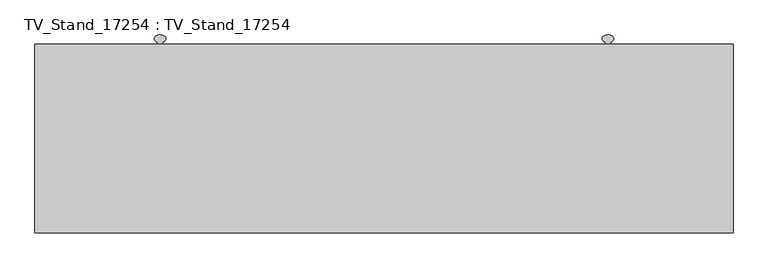
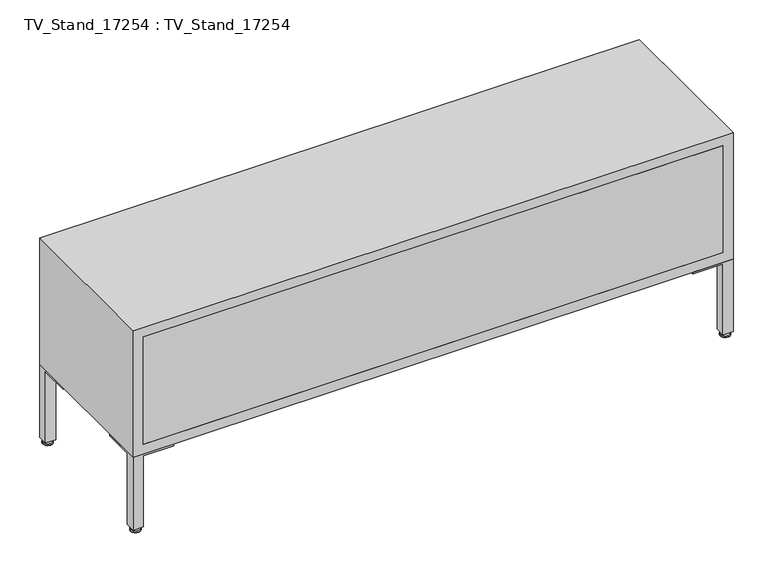
"""IFC4 building model written with IfcOpenShell, lengths in millimetres: furniture geometry, TV_Stand_17254 : TV_Stand_17254."""

from ifc_helpers import new_model, si_unit, point, frame, origin, place, context, project, spatial, polyline, circle_curve, ellipse_curve, trimmed, outline, extrude, source, transform, mapped, element, save
from ifc_brep_helpers import plane_surface, cylinder_surface, revolved_surface, extruded_surface, advanced_brep


def tv_stand_17254_tv_stand_17254_2bb553a4(model_context):
    return source(origin(), model_context, "Body", "SolidModel", [
        extrude(outline(polyline([(530.0, 740.0), (530.0, -740.0), (200.0, -740.0), (200.0, 740.0), (530.0, 740.0)]), holes=[polyline([(505.0, 715.0), (225.0, 715.0), (225.0, -715.0), (505.0, -715.0), (505.0, 715.0)])]), frame((0.0, 0.0, 0.0), z_axis=(0.0, 1.0, 0.0), x_axis=(0.0, 0.0, 1.0)), (0.0, 0.0, 1.0), 400.0),
        extrude(outline(polyline([(-400.0, 12.0), (-412.0, 12.0), (-412.0, 390.0), (-400.0, 390.0), (-400.0, 12.0)])), frame((0.0, 0.0, 225.0), z_axis=(0.0, 0.0, 1.0), x_axis=(1.0, 0.0, 0.0)), (0.0, 0.0, 1.0), 280.0),
        extrude(outline(polyline([(412.0, 12.0), (400.0, 12.0), (400.0, 390.0), (412.0, 390.0), (412.0, 12.0)])), frame((0.0, 0.0, 225.0), z_axis=(0.0, 0.0, 1.0), x_axis=(1.0, 0.0, 0.0)), (0.0, 0.0, 1.0), 280.0),
        extrude(outline(polyline([(715.0, 0.0), (-715.0, 0.0), (-715.0, 12.0), (715.0, 12.0), (715.0, 0.0)])), frame((0.0, 0.0, 225.0), z_axis=(0.0, 0.0, 1.0), x_axis=(1.0, 0.0, 0.0)), (0.0, 0.0, 1.0), 280.0),
        extrude(outline(polyline([(-400.0, 400.0), (-400.0, 390.0), (-713.0, 390.0), (-713.0, 400.0), (-400.0, 400.0)])), frame((0.0, 0.0, 227.0), z_axis=(0.0, 0.0, 1.0), x_axis=(1.0, 0.0, 0.0)), (0.0, 0.0, 1.0), 276.0),
        extrude(outline(polyline([(400.0, 400.0), (713.0, 400.0), (713.0, 390.0), (400.0, 390.0), (400.0, 400.0)])), frame((0.0, 0.0, 227.0), z_axis=(0.0, 0.0, 1.0), x_axis=(1.0, 0.0, 0.0)), (0.0, 0.0, 1.0), 276.0),
        extrude(outline(polyline([(400.0, 12.0), (-400.0, 12.0), (-400.0, 390.0), (400.0, 390.0), (400.0, 12.0)])), frame((0.0, 0.0, 352.5), z_axis=(0.0, 0.0, 1.0), x_axis=(1.0, 0.0, 0.0)), (0.0, 0.0, 1.0), 25.0),
        advanced_brep(
        [(-715.0, 400.0, 10.0), (-715.0, 375.0, 10.0), (-740.0, 375.0, 10.0), (-740.0, 400.0, 10.0), (-730.0, 387.5, 10.0), (-725.0, 387.5, 10.0), (-740.0, 400.0, 200.0), (-640.0, 400.0, 200.0), (-640.0, 400.0, 195.0), (-715.0, 400.0, 195.0), (-740.0, 375.0, 195.0), (-740.0, 300.0, 195.0), (-740.0, 300.0, 200.0), (-715.0, 375.0, 195.0), (-715.0, 300.0, 200.0), (-715.0, 375.0, 200.0), (-640.0, 375.0, 200.0), (-640.0, 375.0, 195.0), (-715.0, 300.0, 195.0), (-730.0, 387.5, 7.0), (-725.0, 387.5, 7.0), (-738.4284767, 387.5, 3.6286093), (-716.5715233, 387.5, 3.6286093), (-740.0, 387.5, 1.3074176), (-715.0, 387.5, 1.3074176), (-740.0, 387.5, 0.0), (-715.0, 387.5, 0.0), (-727.5, 387.5, 0.0)],
        [
            (0, 1),
            (1, 2),
            (2, 3),
            (3, 0),
            (4, 5, circle_curve(frame((-727.5, 387.5, 10.0), z_axis=(0.0, 0.0, 1.0), x_axis=(-1.0, 0.0, 0.0)), 2.5)),
            (5, 4, circle_curve(frame((-727.5, 387.5, 10.0), z_axis=(0.0, 0.0, 1.0), x_axis=(-1.0, 0.0, 0.0)), 2.5)),
            (3, 6),
            (6, 7),
            (7, 8),
            (8, 9),
            (9, 0),
            (2, 10),
            (10, 11),
            (11, 12),
            (12, 6),
            (1, 13),
            (13, 10),
            (9, 13),
            (12, 14),
            (14, 15),
            (15, 16),
            (16, 7),
            (8, 17),
            (17, 13),
            (13, 18),
            (18, 11),
            (18, 14),
            (13, 15),
            (17, 16),
            (4, 19),
            (19, 20, circle_curve(frame((-727.5, 387.5, 7.0), z_axis=(0.0, 0.0, 1.0), x_axis=(-1.0, 0.0, 0.0)), 2.5)),
            (20, 5),
            (20, 19, circle_curve(frame((-727.5, 387.5, 7.0), z_axis=(0.0, 0.0, 1.0), x_axis=(-1.0, 0.0, 0.0)), 2.5)),
            (19, 21),
            (21, 22, circle_curve(frame((-727.5, 387.5, 3.6286093), z_axis=(0.0, 0.0, 1.0), x_axis=(-1.0, 0.0, 0.0)), 10.9284767)),
            (22, 20),
            (22, 21, circle_curve(frame((-727.5, 387.5, 3.6286093), z_axis=(0.0, 0.0, 1.0), x_axis=(-1.0, 0.0, 0.0)), 10.9284767)),
            (21, 23, circle_curve(frame((-737.5, 387.5, 1.3074176), z_axis=(0.0, -1.0, 0.0), x_axis=(1.0, 0.0, 0.0)), 2.5)),
            (23, 24, circle_curve(frame((-727.5, 387.5, 1.3074176), z_axis=(0.0, 0.0, 1.0), x_axis=(-1.0, 0.0, 0.0)), 12.5)),
            (24, 22, circle_curve(frame((-717.5, 387.5, 1.3074176), z_axis=(0.0, -1.0, 0.0), x_axis=(-1.0, 0.0, 0.0)), 2.5)),
            (24, 23, circle_curve(frame((-727.5, 387.5, 1.3074176), z_axis=(0.0, 0.0, 1.0), x_axis=(-1.0, 0.0, 0.0)), 12.5)),
            (23, 25),
            (25, 26, circle_curve(frame((-727.5, 387.5, 0.0), z_axis=(0.0, 0.0, 1.0), x_axis=(-1.0, 0.0, 0.0)), 12.5)),
            (26, 24),
            (26, 25, circle_curve(frame((-727.5, 387.5, 0.0), z_axis=(0.0, 0.0, 1.0), x_axis=(-1.0, 0.0, 0.0)), 12.5)),
            (25, 27),
            (27, 26),
        ],
        [
            plane_surface(frame((-740.0, 400.0, 10.0), z_axis=(0.0, 0.0, -1.0), x_axis=(1.0, 0.0, 0.0))),
            plane_surface(frame((-715.0, 400.0, 195.0), z_axis=(0.0, 1.0, 0.0), x_axis=(0.0, 0.0, -1.0))),
            plane_surface(frame((-740.0, 400.0, 195.0), z_axis=(-1.0, 0.0, 0.0), x_axis=(0.0, 0.0, -1.0))),
            plane_surface(frame((-740.0, 375.0, 195.0), z_axis=(0.0, -1.0, 0.0), x_axis=(0.0, 0.0, -1.0))),
            plane_surface(frame((-715.0, 375.0, 195.0), z_axis=(1.0, 0.0, 0.0), x_axis=(0.0, 0.0, -1.0))),
            plane_surface(frame((-740.0, 300.0, 200.0), z_axis=(0.0, 0.0, 1.0), x_axis=(1.0, 0.0, 0.0))),
            plane_surface(frame((-740.0, 300.0, 195.0), z_axis=(0.0, 0.0, -1.0), x_axis=(-1.0, 0.0, 0.0))),
            plane_surface(frame((-740.0, 300.0, 200.0), z_axis=(0.0, -1.0, 0.0), x_axis=(0.0, 0.0, -1.0))),
            plane_surface(frame((-715.0, 300.0, 200.0), z_axis=(1.0, 0.0, 0.0), x_axis=(0.0, 0.0, -1.0))),
            plane_surface(frame((-715.0, 375.0, 200.0), z_axis=(0.0, -1.0, 0.0), x_axis=(0.0, 0.0, -1.0))),
            plane_surface(frame((-640.0, 375.0, 200.0), z_axis=(1.0, 0.0, 0.0), x_axis=(0.0, 0.0, -1.0))),
            cylinder_surface(frame((-727.5, 387.5, 10.0), z_axis=(0.0, 0.0, 1.0), x_axis=(-1.0, 0.0, 0.0)), 2.5),
            revolved_surface(polyline([(-738.4284767, 387.5, 3.6286093), (-730.0, 387.5, 7.0)]), (-727.5, 387.5, 10.0), (0.0, 0.0, 1.0)),
            revolved_surface(trimmed(ellipse_curve(frame((-737.5, 387.5, 1.3074176), z_axis=(0.0, 1.0, 0.0), x_axis=(1.0, 0.0, 0.0)), 2.5, 2.5), [point((-740.0, 387.5, 1.3074176))], [point((-738.4284767, 387.5, 3.6286093))], True, "CARTESIAN"), (-727.5, 387.5, 10.0), (0.0, 0.0, 1.0)),
            cylinder_surface(frame((-727.5, 387.5, 10.0), z_axis=(0.0, 0.0, 1.0), x_axis=(-1.0, 0.0, 0.0)), 12.5),
            plane_surface(frame((-727.5, 387.5, 0.0), z_axis=(0.0, 0.0, -1.0), x_axis=(-1.0, 0.0, 0.0))),
        ],
        [
            (0, [[1, 2, 3, 4], [5, 6]]),
            (1, [[-4, 7, 8, 9, 10, 11]]),
            (2, [[-3, 12, 13, 14, 15, -7]]),
            (3, [[-2, 16, 17, -12]]),
            (4, [[-1, -11, 18, -16]]),
            (5, [[19, 20, 21, 22, -8, -15]]),
            (6, [[23, 24, -18, -10]]),
            (6, [[25, 26, -13, -17]]),
            (7, [[-19, -14, -26, 27]]),
            (8, [[-20, -27, -25, 28]]),
            (9, [[-21, -28, -24, 29]]),
            (10, [[-22, -29, -23, -9]]),
            (11, [[30, 31, 32, -5]]),
            (11, [[-30, -6, -32, 33]]),
            (12, [[-31, 34, 35, 36]]),
            (12, [[-33, -36, 37, -34]]),
            (13, [[-35, 38, 39, 40]]),
            (13, [[-37, -40, 41, -38]]),
            (14, [[-39, 42, 43, 44]]),
            (14, [[-41, -44, 45, -42]]),
            (15, [[-43, 46, 47]]),
            (15, [[-45, -47, -46]]),
        ],
    ),
        advanced_brep(
        [(-715.0, 0.0, 10.0), (-740.0, 0.0, 10.0), (-740.0, 25.0, 10.0), (-715.0, 25.0, 10.0), (-725.0, 12.5, 10.0), (-730.0, 12.5, 10.0), (-715.0, 25.0, 195.0), (-715.0, 0.0, 195.0), (-740.0, 25.0, 195.0), (-740.0, 0.0, 200.0), (-740.0, 100.0, 200.0), (-740.0, 100.0, 195.0), (-640.0, 0.0, 195.0), (-640.0, 0.0, 200.0), (-640.0, 25.0, 200.0), (-715.0, 25.0, 200.0), (-715.0, 100.0, 200.0), (-715.0, 100.0, 195.0), (-640.0, 25.0, 195.0), (-725.0, 12.5, 7.0), (-730.0, 12.5, 7.0), (-716.5715233, 12.5, 3.6286093), (-738.4284767, 12.5, 3.6286093), (-715.0, 12.5, 1.3074176), (-740.0, 12.5, 1.3074176), (-715.0, 12.5, 0.0), (-740.0, 12.5, 0.0), (-727.5, 12.5, 0.0)],
        [
            (0, 1),
            (1, 2),
            (2, 3),
            (3, 0),
            (4, 5, circle_curve(frame((-727.5, 12.5, 10.0), z_axis=(0.0, 0.0, 1.0), x_axis=(-1.0, 0.0, 0.0)), 2.5)),
            (5, 4, circle_curve(frame((-727.5, 12.5, 10.0), z_axis=(0.0, 0.0, 1.0), x_axis=(-1.0, 0.0, 0.0)), 2.5)),
            (3, 6),
            (6, 7),
            (7, 0),
            (2, 8),
            (8, 6),
            (1, 9),
            (9, 10),
            (10, 11),
            (11, 8),
            (7, 12),
            (12, 13),
            (13, 9),
            (13, 14),
            (14, 15),
            (15, 16),
            (16, 10),
            (11, 17),
            (17, 6),
            (6, 18),
            (18, 12),
            (18, 14),
            (6, 15),
            (17, 16),
            (19, 20, circle_curve(frame((-727.5, 12.5, 7.0), z_axis=(0.0, 0.0, 1.0), x_axis=(-1.0, 0.0, 0.0)), 2.5)),
            (20, 5),
            (4, 19),
            (20, 19, circle_curve(frame((-727.5, 12.5, 7.0), z_axis=(0.0, 0.0, 1.0), x_axis=(-1.0, 0.0, 0.0)), 2.5)),
            (19, 21),
            (21, 22, circle_curve(frame((-727.5, 12.5, 3.6286093), z_axis=(0.0, 0.0, 1.0), x_axis=(-1.0, 0.0, 0.0)), 10.9284767)),
            (22, 20),
            (22, 21, circle_curve(frame((-727.5, 12.5, 3.6286093), z_axis=(0.0, 0.0, 1.0), x_axis=(-1.0, 0.0, 0.0)), 10.9284767)),
            (21, 23, circle_curve(frame((-717.5, 12.5, 1.3074176), z_axis=(0.0, 1.0, 0.0), x_axis=(-1.0, 0.0, 0.0)), 2.5)),
            (23, 24, circle_curve(frame((-727.5, 12.5, 1.3074176), z_axis=(0.0, 0.0, 1.0), x_axis=(-1.0, 0.0, 0.0)), 12.5)),
            (24, 22, circle_curve(frame((-737.5, 12.5, 1.3074176), z_axis=(0.0, 1.0, 0.0), x_axis=(1.0, 0.0, 0.0)), 2.5)),
            (24, 23, circle_curve(frame((-727.5, 12.5, 1.3074176), z_axis=(0.0, 0.0, 1.0), x_axis=(-1.0, 0.0, 0.0)), 12.5)),
            (23, 25),
            (25, 26, circle_curve(frame((-727.5, 12.5, 0.0), z_axis=(0.0, 0.0, 1.0), x_axis=(-1.0, 0.0, 0.0)), 12.5)),
            (26, 24),
            (26, 25, circle_curve(frame((-727.5, 12.5, 0.0), z_axis=(0.0, 0.0, 1.0), x_axis=(-1.0, 0.0, 0.0)), 12.5)),
            (25, 27),
            (27, 26),
        ],
        [
            plane_surface(frame((-740.0, 400.0, 10.0), z_axis=(0.0, 0.0, -1.0), x_axis=(1.0, 0.0, 0.0))),
            plane_surface(frame((-715.0, 0.0, 195.0), z_axis=(1.0, 0.0, 0.0), x_axis=(0.0, 0.0, -1.0))),
            plane_surface(frame((-715.0, 25.0, 195.0), z_axis=(0.0, 1.0, 0.0), x_axis=(0.0, 0.0, -1.0))),
            plane_surface(frame((-740.0, 25.0, 195.0), z_axis=(-1.0, 0.0, 0.0), x_axis=(0.0, 0.0, -1.0))),
            plane_surface(frame((-740.0, 0.0, 195.0), z_axis=(0.0, -1.0, 0.0), x_axis=(0.0, 0.0, -1.0))),
            plane_surface(frame((-740.0, 300.0, 200.0), z_axis=(0.0, 0.0, 1.0), x_axis=(1.0, 0.0, 0.0))),
            plane_surface(frame((-740.0, 300.0, 195.0), z_axis=(0.0, 0.0, -1.0), x_axis=(-1.0, 0.0, 0.0))),
            plane_surface(frame((-640.0, 0.0, 200.0), z_axis=(1.0, 0.0, 0.0), x_axis=(0.0, 0.0, -1.0))),
            plane_surface(frame((-640.0, 25.0, 200.0), z_axis=(0.0, 1.0, 0.0), x_axis=(0.0, 0.0, -1.0))),
            plane_surface(frame((-715.0, 25.0, 200.0), z_axis=(1.0, 0.0, 0.0), x_axis=(0.0, 0.0, -1.0))),
            plane_surface(frame((-715.0, 100.0, 200.0), z_axis=(0.0, 1.0, 0.0), x_axis=(0.0, 0.0, -1.0))),
            cylinder_surface(frame((-727.5, 12.5, 10.0), z_axis=(0.0, 0.0, -1.0), x_axis=(-1.0, 0.0, 0.0)), 2.5),
            revolved_surface(polyline([(-730.0, 12.5, 7.0), (-738.4284767, 12.5, 3.6286093)]), (-727.5, 12.5, 10.0), (0.0, 0.0, -1.0)),
            revolved_surface(trimmed(ellipse_curve(frame((-737.5, 12.5, 1.3074176), z_axis=(0.0, -1.0, 0.0), x_axis=(1.0, 0.0, 0.0)), 2.5, 2.5), [point((-738.4284767, 12.5, 3.6286093))], [point((-740.0, 12.5, 1.3074176))], True, "CARTESIAN"), (-727.5, 12.5, 10.0), (0.0, 0.0, -1.0)),
            cylinder_surface(frame((-727.5, 12.5, 10.0), z_axis=(0.0, 0.0, -1.0), x_axis=(-1.0, 0.0, 0.0)), 12.5),
            plane_surface(frame((-727.5, 12.5, 0.0), z_axis=(0.0, 0.0, -1.0), x_axis=(-1.0, 0.0, 0.0))),
        ],
        [
            (0, [[1, 2, 3, 4], [5, 6]]),
            (1, [[-4, 7, 8, 9]]),
            (2, [[-3, 10, 11, -7]]),
            (3, [[-2, 12, 13, 14, 15, -10]]),
            (4, [[-1, -9, 16, 17, 18, -12]]),
            (5, [[-13, -18, 19, 20, 21, 22]]),
            (6, [[23, 24, -11, -15]]),
            (6, [[25, 26, -16, -8]]),
            (7, [[-19, -17, -26, 27]]),
            (8, [[-20, -27, -25, 28]]),
            (9, [[-21, -28, -24, 29]]),
            (10, [[-22, -29, -23, -14]]),
            (11, [[30, 31, -5, 32]]),
            (11, [[-31, 33, -32, -6]]),
            (12, [[-30, 34, 35, 36]]),
            (12, [[-33, -36, 37, -34]]),
            (13, [[-35, 38, 39, 40]]),
            (13, [[-37, -40, 41, -38]]),
            (14, [[-39, 42, 43, 44]]),
            (14, [[-41, -44, 45, -42]]),
            (15, [[-43, 46, 47]]),
            (15, [[-45, -47, -46]]),
        ],
    ),
        advanced_brep(
        [(715.0, 400.0, 10.0), (740.0, 400.0, 10.0), (740.0, 375.0, 10.0), (715.0, 375.0, 10.0), (725.0, 387.5, 10.0), (730.0, 387.5, 10.0), (715.0, 375.0, 195.0), (715.0, 400.0, 195.0), (740.0, 375.0, 195.0), (740.0, 400.0, 200.0), (740.0, 300.0, 200.0), (740.0, 300.0, 195.0), (640.0, 400.0, 195.0), (640.0, 400.0, 200.0), (640.0, 375.0, 200.0), (715.0, 375.0, 200.0), (715.0, 300.0, 200.0), (715.0, 300.0, 195.0), (640.0, 375.0, 195.0), (725.0, 387.5, 7.0), (730.0, 387.5, 7.0), (716.5715233, 387.5, 3.6286093), (738.4284767, 387.5, 3.6286093), (715.0, 387.5, 1.3074176), (740.0, 387.5, 1.3074176), (715.0, 387.5, 0.0), (740.0, 387.5, 0.0), (727.5, 387.5, 0.0)],
        [
            (0, 1),
            (1, 2),
            (2, 3),
            (3, 0),
            (4, 5, circle_curve(frame((727.5, 387.5, 10.0), z_axis=(0.0, 0.0, 1.0), x_axis=(1.0, 0.0, 0.0)), 2.5)),
            (5, 4, circle_curve(frame((727.5, 387.5, 10.0), z_axis=(0.0, 0.0, 1.0), x_axis=(1.0, 0.0, 0.0)), 2.5)),
            (3, 6),
            (6, 7),
            (7, 0),
            (2, 8),
            (8, 6),
            (1, 9),
            (9, 10),
            (10, 11),
            (11, 8),
            (7, 12),
            (12, 13),
            (13, 9),
            (13, 14),
            (14, 15),
            (15, 16),
            (16, 10),
            (11, 17),
            (17, 6),
            (6, 18),
            (18, 12),
            (18, 14),
            (6, 15),
            (17, 16),
            (19, 20, circle_curve(frame((727.5, 387.5, 7.0), z_axis=(0.0, 0.0, 1.0), x_axis=(1.0, 0.0, 0.0)), 2.5)),
            (20, 5),
            (4, 19),
            (20, 19, circle_curve(frame((727.5, 387.5, 7.0), z_axis=(0.0, 0.0, 1.0), x_axis=(1.0, 0.0, 0.0)), 2.5)),
            (19, 21),
            (21, 22, circle_curve(frame((727.5, 387.5, 3.6286093), z_axis=(0.0, 0.0, 1.0), x_axis=(1.0, 0.0, 0.0)), 10.9284767)),
            (22, 20),
            (22, 21, circle_curve(frame((727.5, 387.5, 3.6286093), z_axis=(0.0, 0.0, 1.0), x_axis=(1.0, 0.0, 0.0)), 10.9284767)),
            (21, 23, circle_curve(frame((717.5, 387.5, 1.3074176), z_axis=(0.0, -1.0, 0.0), x_axis=(1.0, 0.0, 0.0)), 2.5)),
            (23, 24, circle_curve(frame((727.5, 387.5, 1.3074176), z_axis=(0.0, 0.0, 1.0), x_axis=(1.0, 0.0, 0.0)), 12.5)),
            (24, 22, circle_curve(frame((737.5, 387.5, 1.3074176), z_axis=(0.0, -1.0, 0.0), x_axis=(-1.0, 0.0, 0.0)), 2.5)),
            (24, 23, circle_curve(frame((727.5, 387.5, 1.3074176), z_axis=(0.0, 0.0, 1.0), x_axis=(1.0, 0.0, 0.0)), 12.5)),
            (23, 25),
            (25, 26, circle_curve(frame((727.5, 387.5, 0.0), z_axis=(0.0, 0.0, 1.0), x_axis=(1.0, 0.0, 0.0)), 12.5)),
            (26, 24),
            (26, 25, circle_curve(frame((727.5, 387.5, 0.0), z_axis=(0.0, 0.0, 1.0), x_axis=(1.0, 0.0, 0.0)), 12.5)),
            (25, 27),
            (27, 26),
        ],
        [
            plane_surface(frame((-740.0, 400.0, 10.0), z_axis=(0.0, 0.0, -1.0), x_axis=(1.0, 0.0, 0.0))),
            plane_surface(frame((715.0, 400.0, 195.0), z_axis=(-1.0, 0.0, 0.0), x_axis=(0.0, 0.0, -1.0))),
            plane_surface(frame((715.0, 375.0, 195.0), z_axis=(0.0, -1.0, 0.0), x_axis=(0.0, 0.0, -1.0))),
            plane_surface(frame((740.0, 375.0, 195.0), z_axis=(1.0, 0.0, 0.0), x_axis=(0.0, 0.0, -1.0))),
            plane_surface(frame((740.0, 400.0, 195.0), z_axis=(0.0, 1.0, 0.0), x_axis=(0.0, 0.0, -1.0))),
            plane_surface(frame((-740.0, 300.0, 200.0), z_axis=(0.0, 0.0, 1.0), x_axis=(1.0, 0.0, 0.0))),
            plane_surface(frame((-740.0, 300.0, 195.0), z_axis=(0.0, 0.0, -1.0), x_axis=(-1.0, 0.0, 0.0))),
            plane_surface(frame((640.0, 400.0, 200.0), z_axis=(-1.0, 0.0, 0.0), x_axis=(0.0, 0.0, -1.0))),
            plane_surface(frame((640.0, 375.0, 200.0), z_axis=(0.0, -1.0, 0.0), x_axis=(0.0, 0.0, -1.0))),
            plane_surface(frame((715.0, 375.0, 200.0), z_axis=(-1.0, 0.0, 0.0), x_axis=(0.0, 0.0, -1.0))),
            plane_surface(frame((715.0, 300.0, 200.0), z_axis=(0.0, -1.0, 0.0), x_axis=(0.0, 0.0, -1.0))),
            cylinder_surface(frame((727.5, 387.5, 10.0), z_axis=(0.0, 0.0, -1.0), x_axis=(1.0, 0.0, 0.0)), 2.5),
            revolved_surface(polyline([(730.0, 387.5, 7.0), (738.4284767, 387.5, 3.6286093)]), (727.5, 387.5, 10.0), (0.0, 0.0, -1.0)),
            revolved_surface(trimmed(ellipse_curve(frame((737.5, 387.5, 1.3074176), z_axis=(0.0, 1.0, 0.0), x_axis=(-1.0, 0.0, 0.0)), 2.5, 2.5), [point((738.4284767, 387.5, 3.6286093))], [point((740.0, 387.5, 1.3074176))], True, "CARTESIAN"), (727.5, 387.5, 10.0), (0.0, 0.0, -1.0)),
            cylinder_surface(frame((727.5, 387.5, 10.0), z_axis=(0.0, 0.0, -1.0), x_axis=(1.0, 0.0, 0.0)), 12.5),
            plane_surface(frame((727.5, 387.5, 0.0), z_axis=(0.0, 0.0, -1.0), x_axis=(1.0, 0.0, 0.0))),
        ],
        [
            (0, [[1, 2, 3, 4], [5, 6]]),
            (1, [[-4, 7, 8, 9]]),
            (2, [[-3, 10, 11, -7]]),
            (3, [[-2, 12, 13, 14, 15, -10]]),
            (4, [[-1, -9, 16, 17, 18, -12]]),
            (5, [[-13, -18, 19, 20, 21, 22]]),
            (6, [[23, 24, -11, -15]]),
            (6, [[25, 26, -16, -8]]),
            (7, [[-19, -17, -26, 27]]),
            (8, [[-20, -27, -25, 28]]),
            (9, [[-21, -28, -24, 29]]),
            (10, [[-22, -29, -23, -14]]),
            (11, [[30, 31, -5, 32]]),
            (11, [[-31, 33, -32, -6]]),
            (12, [[-30, 34, 35, 36]]),
            (12, [[-33, -36, 37, -34]]),
            (13, [[-35, 38, 39, 40]]),
            (13, [[-37, -40, 41, -38]]),
            (14, [[-39, 42, 43, 44]]),
            (14, [[-41, -44, 45, -42]]),
            (15, [[-43, 46, 47]]),
            (15, [[-45, -47, -46]]),
        ],
    ),
        advanced_brep(
        [(715.0, 0.0, 10.0), (715.0, 25.0, 10.0), (740.0, 25.0, 10.0), (740.0, 0.0, 10.0), (730.0, 12.5, 10.0), (725.0, 12.5, 10.0), (740.0, 0.0, 200.0), (640.0, 0.0, 200.0), (640.0, 0.0, 195.0), (715.0, 0.0, 195.0), (740.0, 25.0, 195.0), (740.0, 100.0, 195.0), (740.0, 100.0, 200.0), (715.0, 25.0, 195.0), (715.0, 100.0, 200.0), (715.0, 25.0, 200.0), (640.0, 25.0, 200.0), (640.0, 25.0, 195.0), (715.0, 100.0, 195.0), (730.0, 12.5, 7.0), (725.0, 12.5, 7.0), (738.4284767, 12.5, 3.6286093), (716.5715233, 12.5, 3.6286093), (740.0, 12.5, 1.3074176), (715.0, 12.5, 1.3074176), (740.0, 12.5, 0.0), (715.0, 12.5, 0.0), (727.5, 12.5, 0.0)],
        [
            (0, 1),
            (1, 2),
            (2, 3),
            (3, 0),
            (4, 5, circle_curve(frame((727.5, 12.5, 10.0), z_axis=(0.0, 0.0, 1.0), x_axis=(1.0, 0.0, 0.0)), 2.5)),
            (5, 4, circle_curve(frame((727.5, 12.5, 10.0), z_axis=(0.0, 0.0, 1.0), x_axis=(1.0, 0.0, 0.0)), 2.5)),
            (3, 6),
            (6, 7),
            (7, 8),
            (8, 9),
            (9, 0),
            (2, 10),
            (10, 11),
            (11, 12),
            (12, 6),
            (1, 13),
            (13, 10),
            (9, 13),
            (12, 14),
            (14, 15),
            (15, 16),
            (16, 7),
            (8, 17),
            (17, 13),
            (13, 18),
            (18, 11),
            (18, 14),
            (13, 15),
            (17, 16),
            (4, 19),
            (19, 20, circle_curve(frame((727.5, 12.5, 7.0), z_axis=(0.0, 0.0, 1.0), x_axis=(1.0, 0.0, 0.0)), 2.5)),
            (20, 5),
            (20, 19, circle_curve(frame((727.5, 12.5, 7.0), z_axis=(0.0, 0.0, 1.0), x_axis=(1.0, 0.0, 0.0)), 2.5)),
            (19, 21),
            (21, 22, circle_curve(frame((727.5, 12.5, 3.6286093), z_axis=(0.0, 0.0, 1.0), x_axis=(1.0, 0.0, 0.0)), 10.9284767)),
            (22, 20),
            (22, 21, circle_curve(frame((727.5, 12.5, 3.6286093), z_axis=(0.0, 0.0, 1.0), x_axis=(1.0, 0.0, 0.0)), 10.9284767)),
            (21, 23, circle_curve(frame((737.5, 12.5, 1.3074176), z_axis=(0.0, 1.0, 0.0), x_axis=(-1.0, 0.0, 0.0)), 2.5)),
            (23, 24, circle_curve(frame((727.5, 12.5, 1.3074176), z_axis=(0.0, 0.0, 1.0), x_axis=(1.0, 0.0, 0.0)), 12.5)),
            (24, 22, circle_curve(frame((717.5, 12.5, 1.3074176), z_axis=(0.0, 1.0, 0.0), x_axis=(1.0, 0.0, 0.0)), 2.5)),
            (24, 23, circle_curve(frame((727.5, 12.5, 1.3074176), z_axis=(0.0, 0.0, 1.0), x_axis=(1.0, 0.0, 0.0)), 12.5)),
            (23, 25),
            (25, 26, circle_curve(frame((727.5, 12.5, 0.0), z_axis=(0.0, 0.0, 1.0), x_axis=(1.0, 0.0, 0.0)), 12.5)),
            (26, 24),
            (26, 25, circle_curve(frame((727.5, 12.5, 0.0), z_axis=(0.0, 0.0, 1.0), x_axis=(1.0, 0.0, 0.0)), 12.5)),
            (25, 27),
            (27, 26),
        ],
        [
            plane_surface(frame((-740.0, 400.0, 10.0), z_axis=(0.0, 0.0, -1.0), x_axis=(1.0, 0.0, 0.0))),
            plane_surface(frame((715.0, 0.0, 195.0), z_axis=(0.0, -1.0, 0.0), x_axis=(0.0, 0.0, -1.0))),
            plane_surface(frame((740.0, 0.0, 195.0), z_axis=(1.0, 0.0, 0.0), x_axis=(0.0, 0.0, -1.0))),
            plane_surface(frame((740.0, 25.0, 195.0), z_axis=(0.0, 1.0, 0.0), x_axis=(0.0, 0.0, -1.0))),
            plane_surface(frame((715.0, 25.0, 195.0), z_axis=(-1.0, 0.0, 0.0), x_axis=(0.0, 0.0, -1.0))),
            plane_surface(frame((-740.0, 300.0, 200.0), z_axis=(0.0, 0.0, 1.0), x_axis=(1.0, 0.0, 0.0))),
            plane_surface(frame((-740.0, 300.0, 195.0), z_axis=(0.0, 0.0, -1.0), x_axis=(-1.0, 0.0, 0.0))),
            plane_surface(frame((740.0, 100.0, 200.0), z_axis=(0.0, 1.0, 0.0), x_axis=(0.0, 0.0, -1.0))),
            plane_surface(frame((715.0, 100.0, 200.0), z_axis=(-1.0, 0.0, 0.0), x_axis=(0.0, 0.0, -1.0))),
            plane_surface(frame((715.0, 25.0, 200.0), z_axis=(0.0, 1.0, 0.0), x_axis=(0.0, 0.0, -1.0))),
            plane_surface(frame((640.0, 25.0, 200.0), z_axis=(-1.0, 0.0, 0.0), x_axis=(0.0, 0.0, -1.0))),
            cylinder_surface(frame((727.5, 12.5, 10.0), z_axis=(0.0, 0.0, 1.0), x_axis=(1.0, 0.0, 0.0)), 2.5),
            revolved_surface(polyline([(738.4284767, 12.5, 3.6286093), (730.0, 12.5, 7.0)]), (727.5, 12.5, 10.0), (0.0, 0.0, 1.0)),
            revolved_surface(trimmed(ellipse_curve(frame((737.5, 12.5, 1.3074176), z_axis=(0.0, -1.0, 0.0), x_axis=(-1.0, 0.0, 0.0)), 2.5, 2.5), [point((740.0, 12.5, 1.3074176))], [point((738.4284767, 12.5, 3.6286093))], True, "CARTESIAN"), (727.5, 12.5, 10.0), (0.0, 0.0, 1.0)),
            cylinder_surface(frame((727.5, 12.5, 10.0), z_axis=(0.0, 0.0, 1.0), x_axis=(1.0, 0.0, 0.0)), 12.5),
            plane_surface(frame((727.5, 12.5, 0.0), z_axis=(0.0, 0.0, -1.0), x_axis=(1.0, 0.0, 0.0))),
        ],
        [
            (0, [[1, 2, 3, 4], [5, 6]]),
            (1, [[-4, 7, 8, 9, 10, 11]]),
            (2, [[-3, 12, 13, 14, 15, -7]]),
            (3, [[-2, 16, 17, -12]]),
            (4, [[-1, -11, 18, -16]]),
            (5, [[19, 20, 21, 22, -8, -15]]),
            (6, [[23, 24, -18, -10]]),
            (6, [[25, 26, -13, -17]]),
            (7, [[-19, -14, -26, 27]]),
            (8, [[-20, -27, -25, 28]]),
            (9, [[-21, -28, -24, 29]]),
            (10, [[-22, -29, -23, -9]]),
            (11, [[30, 31, 32, -5]]),
            (11, [[-30, -6, -32, 33]]),
            (12, [[-31, 34, 35, 36]]),
            (12, [[-33, -36, 37, -34]]),
            (13, [[-35, 38, 39, 40]]),
            (13, [[-37, -40, 41, -38]]),
            (14, [[-39, 42, 43, 44]]),
            (14, [[-41, -44, 45, -42]]),
            (15, [[-43, 46, 47]]),
            (15, [[-45, -47, -46]]),
        ],
    ),
        advanced_brep(
        [(-481.0, 400.0, 450.0), (-469.0, 400.0, 450.0), (-469.0, 405.0337162, 450.0), (-481.0, 405.2092978, 450.0), (-481.0, 400.0, 300.0), (-481.0, 405.2092978, 300.0), (-469.0, 405.0337162, 300.0), (-469.0, 400.0, 300.0)],
        [
            (0, 1),
            (1, 2),
            (2, 3, ellipse_curve(frame((-474.75, 412.1546464, 450.0), z_axis=(0.0, 0.0, 1.0), x_axis=(-1.0, 0.0, 0.0)), 12.5, 8.0197977)),
            (3, 0),
            (4, 5),
            (5, 6, ellipse_curve(frame((-474.75, 412.1546464, 300.0), z_axis=(0.0, 0.0, -1.0), x_axis=(-1.0, 0.0, 0.0)), 12.5, 8.0197977)),
            (6, 7),
            (7, 4),
            (0, 4),
            (7, 1),
            (6, 2),
            (3, 5),
        ],
        [
            plane_surface(frame((-469.0, 400.0, 450.0), z_axis=(0.0, 0.0, 1.0), x_axis=(1.0, 0.0, 0.0))),
            plane_surface(frame((-469.0, 400.0, 300.0), z_axis=(0.0, 0.0, -1.0), x_axis=(-1.0, 0.0, 0.0))),
            plane_surface(frame((-481.0, 400.0, 450.0), z_axis=(0.0, -1.0, 0.0), x_axis=(0.0, 0.0, -1.0))),
            plane_surface(frame((-469.0, 400.0, 450.0), z_axis=(1.0, 0.0, 0.0), x_axis=(0.0, 0.0, -1.0))),
            plane_surface(frame((-481.0, 405.2092978, 450.0), z_axis=(-1.0, 0.0, 0.0), x_axis=(0.0, 0.0, -1.0))),
            extruded_surface(trimmed(ellipse_curve(frame((-474.75, 412.1546464, 150.0), z_axis=(0.0, 0.0, 1.0), x_axis=(-1.0, 0.0, 0.0)), 12.5, 8.0197977), [point((-469.0, 405.0337162, 150.0))], [point((-481.0, 405.2092978, 150.0))], True, "CARTESIAN"), (0.0, 0.0, 150.0), 150.0),
        ],
        [
            (0, [[1, 2, 3, 4]]),
            (1, [[5, 6, 7, 8]]),
            (2, [[-1, 9, -8, 10]]),
            (3, [[-2, -10, -7, 11]]),
            (4, [[-4, 12, -5, -9]]),
            (5, [[-3, -11, -6, -12]]),
        ],
    ),
        advanced_brep(
        [(481.0, 400.0, 450.0), (481.0, 405.2092978, 450.0), (469.0, 405.0337162, 450.0), (469.0, 400.0, 450.0), (481.0, 400.0, 300.0), (469.0, 400.0, 300.0), (469.0, 405.0337162, 300.0), (481.0, 405.2092978, 300.0)],
        [
            (0, 1),
            (1, 2, ellipse_curve(frame((474.75, 412.1546464, 450.0), z_axis=(0.0, 0.0, 1.0), x_axis=(1.0, 0.0, 0.0)), 12.5, 8.0197977)),
            (2, 3),
            (3, 0),
            (4, 5),
            (5, 6),
            (6, 7, ellipse_curve(frame((474.75, 412.1546464, 300.0), z_axis=(0.0, 0.0, -1.0), x_axis=(1.0, 0.0, 0.0)), 12.5, 8.0197977)),
            (7, 4),
            (3, 5),
            (4, 0),
            (2, 6),
            (7, 1),
        ],
        [
            plane_surface(frame((481.0, 400.0, 450.0), z_axis=(0.0, 0.0, 1.0), x_axis=(0.0, 1.0, 0.0))),
            plane_surface(frame((481.0, 400.0, 300.0), z_axis=(0.0, 0.0, -1.0), x_axis=(0.0, -1.0, 0.0))),
            plane_surface(frame((469.0, 400.0, 450.0), z_axis=(0.0, -1.0, 0.0), x_axis=(0.0, 0.0, -1.0))),
            plane_surface(frame((469.0, 405.0337162, 450.0), z_axis=(-1.0, 0.0, 0.0), x_axis=(0.0, 0.0, -1.0))),
            plane_surface(frame((481.0, 400.0, 450.0), z_axis=(1.0, 0.0, 0.0), x_axis=(0.0, 0.0, -1.0))),
            extruded_surface(trimmed(ellipse_curve(frame((474.75, 412.1546464, 150.0), z_axis=(0.0, 0.0, 1.0), x_axis=(1.0, 0.0, 0.0)), 12.5, 8.0197977), [point((481.0, 405.2092978, 150.0))], [point((469.0, 405.0337162, 150.0))], True, "CARTESIAN"), (0.0, 0.0, 150.0), 150.0),
        ],
        [
            (0, [[1, 2, 3, 4]]),
            (1, [[5, 6, 7, 8]]),
            (2, [[-4, 9, -5, 10]]),
            (3, [[-3, 11, -6, -9]]),
            (4, [[-1, -10, -8, 12]]),
            (5, [[-2, -12, -7, -11]]),
        ],
    ),
    ])


if __name__ == "__main__":
    model = new_model("IFC4")
    model_context = context("Model", 3, world=origin())
    ifc_project = project(units=[si_unit("LENGTHUNIT", "METRE", prefix="MILLI")], contexts=[model_context])
    site = spatial("IfcSite", under=ifc_project)
    building = spatial("IfcBuilding", under=site)
    placement = place(None, origin())
    tv_stand_17254_tv_stand_17254_shape = tv_stand_17254_tv_stand_17254_2bb553a4(model_context)
    element("IfcFurniture", 1, ObjectType="TV_Stand_17254 : TV_Stand_17254", at=placement, inside=building, context=model_context, shape_type="MappedRepresentation", body=[
        mapped(tv_stand_17254_tv_stand_17254_shape, transform((0.0, 0.0, 0.0), x_axis=(1.0, 0.0, 0.0), y_axis=(0.0, 1.0, 0.0), z_axis=(0.0, 0.0, 1.0))),
    ])
    save(model, "model.ifc")

# Revit data of these elements
# Type "TV_Stand_17254 : TV_Stand_17254"
#   URL = "http://www.woodwaves.com/products/modern-tv-stand-terra-mar-clove"
#   Stand Width = 4' - 10.26772"
#   Stand Height = 1' - 8.86614"
#   Cupboard Width = 1' - 1.38583"
#   Modern TV Stand - White Wood = Modern TV Stand - White Wood
#   Modern TV Stand - Semi Polished = Modern TV Stand - Semi Polished
#   Modern TV Stand - Oak Wood = Modern TV Stand - Oak Wood
#   Default Elevation = 0
# Element 1 (IfcFurniture, "TV_Stand_17254 : TV_Stand_17254")
#   Materials on its faces: "Modern TV Stand - Semi Polished", "Modern TV Stand - Oak Wood", "Modern TV Stand - White Wood"
# Materials
#   "Modern TV Stand - White Wood": class "Generic", colour RGB 120 120 120, transparency 0, Cost = 0
#   "Modern TV Stand - Semi Polished": class "Generic", colour RGB 120 120 120, transparency 0, Cost = 0
#   "Modern TV Stand - Oak Wood": class "Generic", colour RGB 120 120 120, transparency 0, Cost = 0
